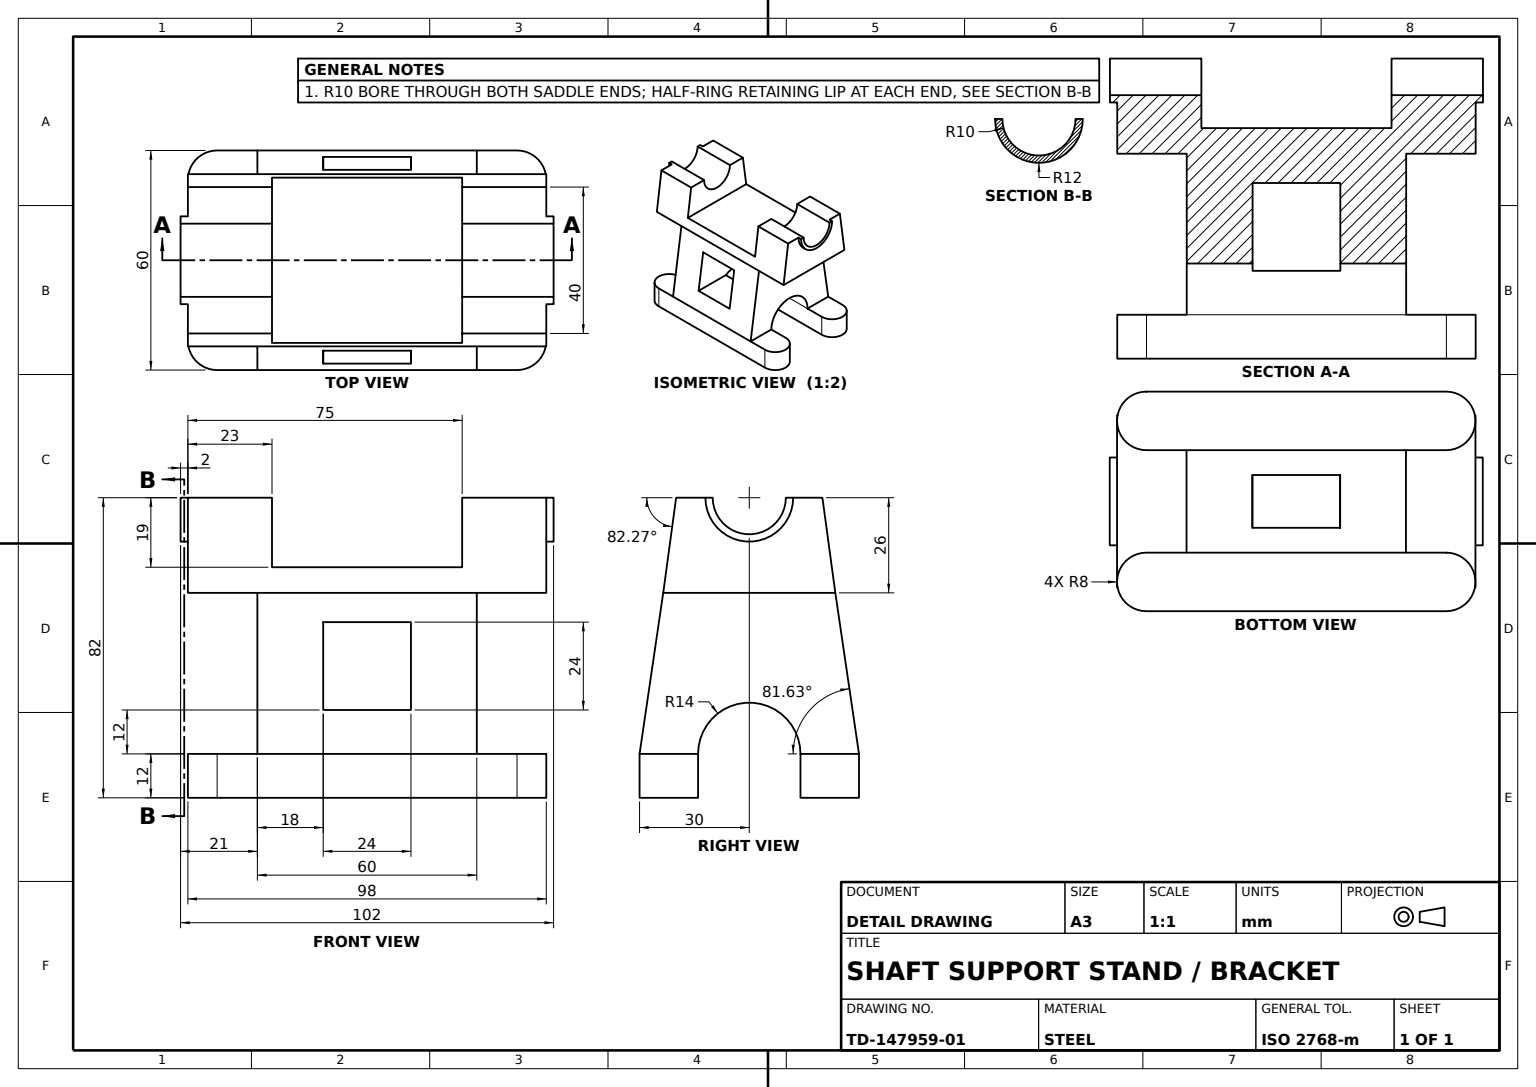
SolidWorks part; units mm, degrees
material "Plain Carbon Steel"
ref_plane "Front Plane" through (0, 0, 0) normal (0, 0, 1) x (1, 0, 0)
ref_plane "Top Plane" through (0, 0, 0) normal (0, 1, 0) x (1, 0, 0)
ref_plane "Right Plane" through (0, 0, 0) normal (1, 0, 0) x (0, 0, -1)
sketch "Base Body Sketch" plane through (0, 0, 0) normal (0, 1, 0) x (1, 0, 0)
  line L1 (-41, -14) -> (41, -14)
  line L2 (41, -30) -> (-41, -30)
  line L3 (41, 30) -> (-41, 30)
  line L4 (-41, 14) -> (41, 14)
  arc A0 (41, 14) -> (41, 30) centre (41, 22) ccw
  arc A1 (-41, 30) -> (-41, 14) centre (-41, 22) ccw
  arc A2 (-41, -30) -> (-41, -14) centre (-41, -22) cw
  arc A3 (41, -14) -> (41, -30) centre (41, -22) cw
  dimension "D1" = 8
  dimension "D2" = 82
  dimension "D5" = 8
  dimension "D11" = 8
  dimension "D3" = 30
  dimension "D4" = 41
  dimension "D6" = 44
  dimension "D7" = 41
  dimension "D8" = 82
  dimension "D9" = 30
  dimension "D10" = 82
  dimension "D12" = 22
  dimension "D13" = 41
  dimension "D14" = 14
extrude "Base Body" add sketch "Base Body Sketch" along normal blind 12
ref_plane "Plane1" through (30, 0, 0) normal (1, 0, 0) x (0, 0, -1)
sketch "Foot Boss Sketch" plane through (30, 0, 0) normal (1, 0, 0) x (0, 0, -1)
  line L1 (-14, 12) -> (-30, 12)
  line L2 (-30, 12) -> (-30, 56)
  line L3 (-30, 56) -> (30, 56)
  line L4 (30, 12) -> (30, 56)
  line L5 (14, 12) -> (30, 12)
  arc A0 (14, 12) -> (-14, 12) centre (0, 12) ccw
  dimension "D1" = 14
  dimension "D2" = 56
extrude "Foot Boss 60" add sketch "Foot Boss Sketch" against normal blind 60
sketch "Window Cut Sketch" plane through (30, 0, 0) normal (1, 0, 0) x (0, 0, -1)
  line L0 (14, 12) -> (30, 12) construction
  line L3 (-23.0834, 59.0332) -> (-30, 12)
  line L4 (23.0834, 59.0332) -> (30, 12)
  line L5 (30, 12) -> (40.9958, 12)
  line L6 (40.9958, 12) -> (40.9958, 59.0332)
  line L7 (40.9958, 59.0332) -> (23.0834, 59.0332)
  line L8 (-33.8353, 59.0332) -> (-33.8353, 12)
  line L9 (-33.8353, 12) -> (-30, 12)
  line L10 (-23.0834, 59.0332) -> (-33.8353, 59.0332)
  line L11 (30, 12) -> (30, 56) construction
  dimension "D1" = 10.9958
  dimension "D2" = 6.9166
  dimension "D3" = 63.8353
  dimension "D4" = 47.0332
extrude "Window Cut" cut sketch "Window Cut Sketch" against normal blind 60
ref_plane "Plane2" through (49, 0, 0) normal (1, 0, 0) x (0, 0, -1)
sketch "Saddle Ends Sketch" plane through (49, 0, 0) normal (1, 0, 0) x (0, 0, -1)
  line L2 (10, 82) -> (20, 82)
  line L3 (20, 82) -> (23.5294, 56)
  line L4 (-10, 82) -> (-20, 82)
  line L5 (-20, 82) -> (-23.5294, 56)
  line L6 (-23.5294, 56) -> (23.5294, 56)
  arc A0 (-10, 82) -> (10, 82) centre (0, 82) ccw
  dimension "D1" = 26
  dimension "D3" = 10
  dimension "D2" = 26
  dimension "D4" = 82
  dimension "D5" = 30.8483
  dimension "D6" = 30.8483
extrude "Saddle Ends 98" add sketch "Saddle Ends Sketch" against normal blind 98
sketch "Saddle Cradle Cut Sketch" plane through (0, 82, 0) normal (0, 1, 0) x (1, 0, 0)
  line L0 (49, -10) -> (49, -20) construction
  line L1 (26, 0) -> (26, -36.491)
  line L2 (26, -36.491) -> (-26, -36.491)
  line L3 (-26, -36.491) -> (-26, 35.7218)
  line L4 (-26, 35.7218) -> (26, 35.7218)
  line L5 (26, 35.7218) -> (26, 0)
  line L6 (-49, -10) -> (49, -10) construction
  dimension "D1" = 23
  dimension "D2" = 75
  dimension "D3" = 10
  dimension "D4" = 45.7218
  dimension "D5" = 26.491
extrude "Saddle Cradle Cut" cut sketch "Saddle Cradle Cut Sketch" against normal blind 19
sketch "Arch Relief Cut Sketch" plane through (0, 0, -30) normal (0, 0, -1) x (-1, 0, 0)
  line L0 (30, 12) -> (-30, 12) construction
  line L1 (0, 24) -> (12, 24)
  line L2 (12, 24) -> (12, 48)
  line L3 (12, 48) -> (-12, 48)
  line L4 (-12, 48) -> (-12, 24)
  line L5 (-12, 24) -> (0, 24)
  dimension "D1" = 29
  dimension "D2" = 41
  dimension "D3" = 12
extrude "Arch Relief Cut" cut sketch "Arch Relief Cut Sketch" against normal blind 93
sketch "Retaining Lip A Sketch" plane through (49, 0, 0) normal (1, 0, 0) x (0, 0, -1)
  line L0 (-12, 82) -> (-10, 82)
  line L1 (10, 82) -> (12, 82)
  arc A0 (-12, 82) -> (12, 82) centre (0, 82) ccw
  arc A1 (-10, 82) -> (10, 82) centre (0, 82) ccw
  dimension "D1" = 12
  dimension "D2" = 10
extrude "Retaining Lip A" add sketch "Retaining Lip A Sketch" along normal blind 2
sketch "Retaining Lip B Sketch" plane through (-49, 0, 0) normal (-1, 0, 0) x (0, 0, 1)
  line L0 (10, 82) -> (12, 82)
  line L1 (-12, 82) -> (-10, 82)
  arc A0 (-10, 82) -> (10, 82) centre (0, 82) ccw
  arc A1 (-12, 82) -> (12, 82) centre (0, 82) ccw
  dimension "D1" = 12
extrude "Retaining Lip B" add sketch "Retaining Lip B Sketch" along normal blind 2
